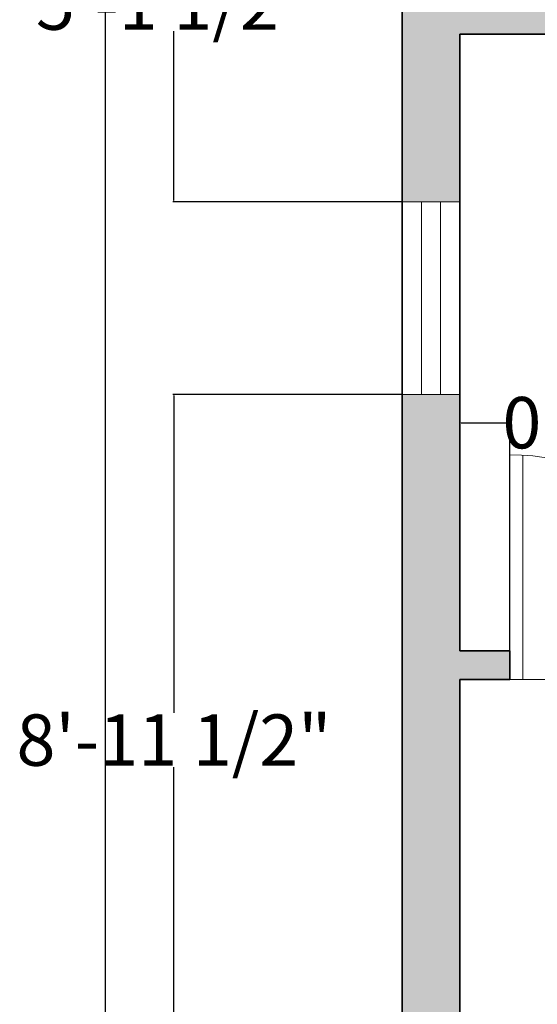
# Model space of a CAD drawing. Units: inches. Extents: x 638 to 1303, y 1 to 699.
# Tile 2 of 21: x 638 to 718, y 156 to 310. Entities that reach past the tile are written whole.
import ezdxf

# ---------------------------------------------------------------- set-up
doc = ezdxf.new("R2010")
doc.units = ezdxf.units.IN
doc.header["$MEASUREMENT"] = 0
for name, color, linetype, lineweight in [('A-ANNO-DIMS', 2, 'Continuous', 18), ('A-DOOR', 4, 'Continuous', 18), ('A-GLAZ', 4, 'Continuous', 18), ('A-WALL', 7, 'Continuous', 35)]:
    doc.layers.add(name, color=color, linetype=linetype, lineweight=lineweight)
doc.layers.add('A-WALL-PATT', color=143, linetype='Continuous', lineweight=13, true_color=0x7aafdf)
doc.styles.get("Standard").update_dxf_attribs({"font": 'arial.ttf'})
doc.dimstyles.get("Standard").update_dxf_attribs({"dimtxt": 8, "dimasz": 0.18, "dimexe": 0.18, "dimexo": 0.0625, "dimgap": 0.09, "dimtad": 0, "dimtih": 1, "dimtoh": 1, "dimdec": 4, "dimzin": 0, "dimdsep": 46, "dimlunit": 3, "dimtxsty": 'Standard', "dimcen": 0.09, "dimadec": 0, "dimazin": 0, "dimtfac": 1, "dimtdec": 4, "dimtofl": 0, "dimtmove": 0, "dimatfit": 3, "dimfxl": 1, "dimtolj": 1, "dimtzin": 0, "dimarcsym": 0})

# ---------------------------------------------------------------- blocks, each defined once
blk = doc.blocks.new('*D1')
at = {"layer": 'A-ANNO-DIMS', "color": 0, "lineweight": -2, "transparency": 16777216}
for p, q in [((697.18, 629.82), (650.92, 629.82)), ((651.1, 629.64), (651.1, 339.99)), ((651.1, 42), (651.1, 331.64)), ((697.18, 41.82), (650.92, 41.82))]:
    blk.add_line(p, q, dxfattribs=at)
at = {"layer": 'A-ANNO-DIMS', "color": 0, "transparency": 16777216}
for points in [[(651.07, 629.64), (651.13, 629.64), (651.1, 629.82)], [(651.07, 42), (651.13, 42), (651.1, 41.82)]]:
    blk.add_solid(points, dxfattribs=at)
at = {"layer": 'Defpoints', "color": 0, "transparency": 16777216}
for p in [(697.24, 629.82), (651.1, 41.82), (697.24, 41.82)]:
    blk.add_point(p, dxfattribs=at)
at = {"layer": 'A-ANNO-DIMS', "color": 0, "transparency": 16777216, "insert": (651.1, 335.82), "char_height": 8, "attachment_point": 5}
blk.add_mtext("\\A1;49'", dxfattribs=at)
blk = doc.blocks.new('DOOR-SWING-35')
for p, q in [((33, 0), (33, 34.94)), ((35, 0), (35, 35)), ((0, 0), (35, 0))]:
    blk.add_line(p, q)
blk.add_arc((35, 0), 35, 90, 180)
blk = doc.blocks.new('WIN-30')
for p, q in [((30, 9), (0, 9)), ((0, 9), (0, 0)), ((30, 0), (30, 9)), ((0, 6), (30, 6)), ((0, 3), (30, 3)), ((0, 0), (30, 0))]:
    blk.add_line(p, q)
blk = doc.blocks.new('*D56')
at = {"layer": 'A-ANNO-DIMS', "color": 0, "lineweight": -2, "transparency": 16777216}
for p, q in [((697.18, 251.22), (661.56, 251.22)), ((661.74, 251.04), (661.74, 201.62)), ((661.74, 143.75), (661.74, 193.17)), ((697.18, 143.57), (661.56, 143.57))]:
    blk.add_line(p, q, dxfattribs=at)
at = {"layer": 'A-ANNO-DIMS', "color": 0, "transparency": 16777216}
for points in [[(661.71, 251.04), (661.77, 251.04), (661.74, 251.22)], [(661.71, 143.75), (661.77, 143.75), (661.74, 143.57)]]:
    blk.add_solid(points, dxfattribs=at)
at = {"layer": 'Defpoints', "color": 0, "transparency": 16777216}
for p in [(661.74, 251.22), (697.24, 251.22), (697.24, 143.57)]:
    blk.add_point(p, dxfattribs=at)
at = {"layer": 'A-ANNO-DIMS', "color": 0, "transparency": 16777216, "insert": (661.74, 197.4), "char_height": 8, "attachment_point": 5}
blk.add_mtext('\\A1;8\'-11 1/2"', dxfattribs=at)
blk = doc.blocks.new('*D57')
at = {"layer": 'A-ANNO-DIMS', "color": 0, "lineweight": -2, "transparency": 16777216}
for p, q in [((697.18, 342.79), (661.56, 342.79)), ((661.74, 342.61), (661.74, 316.23)), ((661.74, 281.4), (661.74, 307.78)), ((697.18, 281.22), (661.56, 281.22))]:
    blk.add_line(p, q, dxfattribs=at)
at = {"layer": 'A-ANNO-DIMS', "color": 0, "transparency": 16777216}
for points in [[(661.71, 342.61), (661.77, 342.61), (661.74, 342.79)], [(661.71, 281.4), (661.77, 281.4), (661.74, 281.22)]]:
    blk.add_solid(points, dxfattribs=at)
at = {"layer": 'Defpoints', "color": 0, "transparency": 16777216}
for p in [(661.74, 342.79), (697.24, 342.79), (697.24, 281.22)]:
    blk.add_point(p, dxfattribs=at)
at = {"layer": 'A-ANNO-DIMS', "color": 0, "transparency": 16777216, "insert": (661.74, 312), "char_height": 8, "attachment_point": 5}
blk.add_mtext('\\A1;5\'-1 1/2"', dxfattribs=at)
blk = doc.blocks.new('*D71')
at = {"layer": 'A-ANNO-DIMS', "color": 0, "lineweight": -2, "transparency": 16777216}
for p, q in [((706.24, 211.38), (706.24, 247)), ((714.01, 211.38), (714.01, 247)), ((706.42, 246.82), (713.83, 246.82)), ((714.01, 246.82), (714.19, 246.82))]:
    blk.add_line(p, q, dxfattribs=at)
at = {"layer": 'A-ANNO-DIMS', "color": 0, "transparency": 16777216}
for points in [[(706.42, 246.85), (706.42, 246.79), (706.24, 246.82)], [(713.83, 246.85), (713.83, 246.79), (714.01, 246.82)]]:
    blk.add_solid(points, dxfattribs=at)
at = {"layer": 'Defpoints', "color": 0, "transparency": 16777216}
for p in [(714.01, 246.82), (706.24, 211.32), (714.01, 211.32)]:
    blk.add_point(p, dxfattribs=at)
at = {"layer": 'A-ANNO-DIMS', "color": 0, "transparency": 16777216, "insert": (724.91, 246.82), "char_height": 8, "attachment_point": 5}
blk.add_mtext('\\A1;0\'-8"', dxfattribs=at)

msp = doc.modelspace()

# ---------------------------------------------------------------- hatches: boundary and pattern name
at = {"layer": 'A-WALL-PATT'}
h = msp.add_hatch(color=256, dxfattribs=at)
h.dxf.hatch_style = 1
h.paths.add_polyline_path([(973.34524, 629.81895), (793.35541, 629.81895), (793.35541, 620.81895), (850.23798, 620.81895), (922.23798, 620.81895), (922.23798, 524.81895), (908.94335, 524.81895), (908.94335, 520.31895), (926.73798, 520.31895), (926.73798, 544.31895), (979.3571, 544.31895), (979.3571, 548.81895), (926.73798, 548.81895), (926.73798, 620.81895), (973.34524, 620.81895)])
h.paths.add_polyline_path([(758.35541, 629.81895), (697.23798, 629.81895), (697.23798, 586.77451), (706.23798, 586.77451), (706.23798, 620.81895), (758.35541, 620.81895)])
h.paths.add_polyline_path([(1075.85281, 629.81895), (1003.34524, 629.81895), (1003.34524, 620.81895), (1046.73798, 620.81895), (1046.73798, 560.81895), (1046.73798, 548.81895), (1026.3571, 548.81895), (1026.3571, 544.31895), (1046.73798, 544.31895), (1046.73798, 486.87457), (1051.23798, 486.87457), (1051.23798, 556.31895), (1162.89753, 556.31895), (1162.89753, 560.81895), (1051.23798, 560.81895), (1051.23798, 620.81895), (1075.85281, 620.81895)])
h.paths.add_polyline_path([(1228.23798, 629.81895), (1105.85281, 629.81895), (1105.85281, 620.81895), (1219.23798, 620.81895), (1219.23798, 560.81895), (1197.89753, 560.81895), (1197.89753, 556.31895), (1219.23798, 556.31895), (1219.23798, 498.80084), (1228.23798, 498.80084)])
h.paths.add_polyline_path([(1051.23798, 439.87457), (1046.73798, 439.87457), (1046.73798, 407.81895), (1219.23798, 407.81895), (1219.23798, 381.66175), (1228.23798, 381.66175), (1228.23798, 451.80084), (1219.23798, 451.80084), (1219.23798, 412.31895), (1051.23798, 412.31895)])
h.paths.add_polyline_path([(1228.23798, 346.66175), (1219.23798, 346.66175), (1219.23798, 335.81895), (1046.73798, 335.81895), (1046.73798, 273.56895), (1051.23798, 273.56895), (1051.23798, 331.31895), (1219.23798, 331.31895), (1219.23798, 308.99654), (1228.23798, 308.99654)])
h.paths.add_polyline_path([(1228.23798, 261.99654), (1219.23798, 261.99654), (1219.23798, 211.31895), (1051.23798, 211.31895), (1051.23798, 226.56895), (1046.73798, 226.56895), (1046.73798, 211.31895), (983.84714, 211.31895), (983.84714, 206.81895), (1219.23798, 206.81895), (1219.23798, 166.83987), (1228.23798, 166.83987)])
h.paths.add_polyline_path([(1228.23798, 119.83987), (1219.23798, 119.83987), (1219.23798, 50.81895), (1197.89277, 50.81895), (1197.89277, 41.81895), (1228.23798, 41.81895)])
h.paths.add_polyline_path([(1162.89277, 50.81895), (1069.02949, 50.81895), (1069.02949, 41.81895), (1162.89277, 41.81895)])
h.paths.add_polyline_path([(1010.02949, 50.81895), (941.89631, 50.81895), (917.77455, 50.81895), (917.77455, 41.81895), (941.89631, 41.81895), (1010.02949, 41.81895)])
h.paths.add_polyline_path([(882.77455, 50.81895), (854.73798, 50.81895), (854.73798, 145.50379), (850.23798, 145.50379), (850.23798, 50.81895), (793.49755, 50.81895), (793.49755, 41.81895), (882.77455, 41.81895)])
h.paths.add_polyline_path([(746.49755, 50.81895), (706.23798, 50.81895), (706.23798, 96.57416), (697.23798, 96.57416), (697.23798, 41.81895), (746.49755, 41.81895)])
h.paths.add_polyline_path([(706.23798, 206.81895), (714.01165, 206.81895), (714.01165, 211.31895), (706.23798, 211.31895), (706.23798, 251.21966), (697.23798, 251.21966), (697.23798, 143.57416), (706.23798, 143.57416)])
h.paths.add_polyline_path([(923.84714, 211.31895), (854.73798, 211.31895), (854.73798, 397.8313), (850.23798, 397.8313), (850.23798, 388.31895), (747.9539, 388.31895), (747.9539, 383.81895), (850.23798, 383.81895), (850.23798, 311.81895), (706.23798, 311.81895), (706.23798, 342.78787), (697.23798, 342.78787), (697.23798, 281.21966), (706.23798, 281.21966), (706.23798, 307.31895), (850.23798, 307.31895), (850.23798, 211.31895), (749.01165, 211.31895), (749.01165, 206.81895), (850.23798, 206.81895), (850.23798, 192.50379), (854.73798, 192.50379), (854.73798, 206.81895), (923.84714, 206.81895)])
h.paths.add_polyline_path([(706.23798, 434.70471), (697.23798, 434.70471), (697.23798, 372.78787), (706.23798, 372.78787), (706.23798, 383.81895), (712.9539, 383.81895), (712.9539, 388.31895), (706.23798, 388.31895)])
h.paths.add_polyline_path([(706.23798, 520.31895), (850.23798, 520.31895), (850.23798, 444.8313), (854.73798, 444.8313), (854.73798, 520.31895), (861.94335, 520.31895), (861.94335, 524.81895), (706.23798, 524.81895), (706.23798, 551.77451), (697.23798, 551.77451), (697.23798, 481.70471), (706.23798, 481.70471)])

# ---------------------------------------------------------------- linework, layer by layer
at = {"layer": 'A-WALL'}
for p, q in [((697.23798, 41.81895), (697.23798, 629.81895)), ((850.23798, 307.31895), (706.23798, 307.31895)), ((706.23798, 211.31895), (706.23798, 307.31895)), ((714.01165, 211.31895), (706.23798, 211.31895)), ((714.01165, 211.31895), (714.01165, 206.81895)), ((706.23798, 50.81895), (706.23798, 206.81895)), ((714.01165, 206.81895), (706.23798, 206.81895))]:
    msp.add_line(p, q, dxfattribs=at)

# ---------------------------------------------------------------- block references
at = {"layer": 'A-DOOR', "extrusion": (0, 0, -1), "zscale": -1}
msp.add_blockref('DOOR-SWING-35', (-749.01118, 206.819), dxfattribs=at)
at = {"layer": 'A-GLAZ', "rotation": 269.9999999999995}
msp.add_blockref('WIN-30', (697.23803, 281.21948), dxfattribs=at)

# ---------------------------------------------------------------- dimensions: what is measured, and where the dimension line sits
at = {"layer": 'A-ANNO-DIMS'}
for base, p1, p2, override, picture, middle in [((651.10111, 41.81895), (697.23798, 629.81895), (697.23798, 41.81895), {"dimclrd": 0, "dimclre": 0, "dimclrt": 0}, '*D1', (651.10111, 335.81895)), ((661.73798, 342.78787), (697.23798, 281.21966), (697.23798, 342.78787), {"dimdec": 1, "dimlfac": 1, "dimrnd": 0, "dimzin": 1, "dimdsep": 46, "dimlunit": 4, "dimfrac": 2}, '*D57', (661.73798, 312.00377)), ((661.73798, 251.21966), (697.23798, 143.57416), (697.23798, 251.21966), {"dimdec": 1, "dimlfac": 1, "dimrnd": 0, "dimzin": 1, "dimdsep": 46, "dimlunit": 4, "dimfrac": 2}, '*D56', (661.73798, 197.39691))]:
    dim = msp.add_linear_dim(base=base, p1=p1, p2=p2, angle=90, dimstyle='Standard', override=override, dxfattribs=at)
    dim.commit()
    dim.dimension.update_dxf_attribs({"geometry": picture, "text_midpoint": middle})
dim = msp.add_linear_dim(base=(714.01165, 246.81895), p1=(706.23798, 211.31895), p2=(714.01165, 211.31895), dimstyle='Standard', override={"dimdec": 1, "dimlfac": 1, "dimrnd": 0, "dimzin": 1, "dimdsep": 46, "dimlunit": 4, "dimfrac": 2}, dxfattribs=at)
dim.commit()
dim.dimension.update_dxf_attribs({"geometry": '*D71', "text_midpoint": (724.91467, 246.81895)})

doc.saveas('drawing.dxf')
